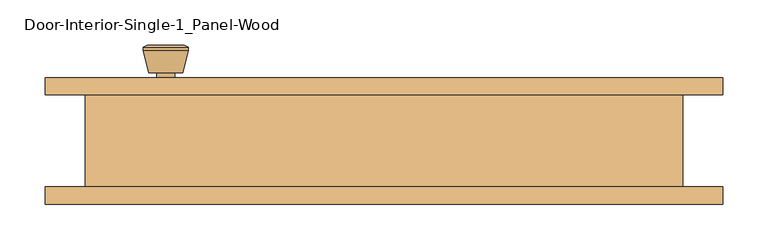
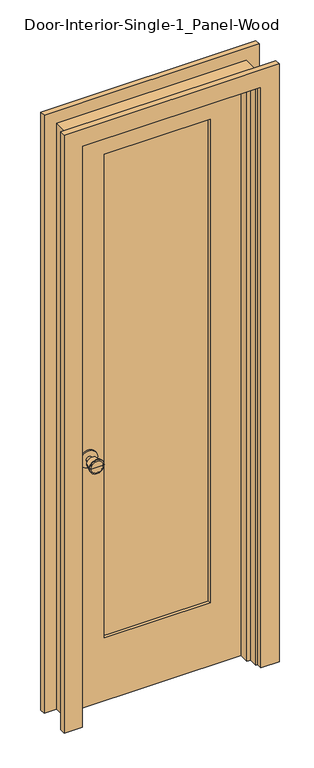
"""IFC4 building model written with IfcOpenShell, lengths in millimetres: door geometry, Door-Interior-Single-1_Panel-Wood."""

from ifc_helpers import new_model, si_unit, point, frame, frame_2d, origin, place, context, project, spatial, polyline, circle_curve, trimmed, segment, composite_curve, outline, extrude, faceted_brep, source, transform, mapped, element, save
from ifc_brep_helpers import plane_surface, cylinder_surface, revolved_surface, advanced_brep


def door_interior_single_1_panel_wood_33af59b7(model_context):
    return source(origin(), model_context, "Body", "SolidModel", [
        advanced_brep(
        [(-241.3, 6.7, 914.4), (-231.3, 6.7, 914.4), (-251.3, 6.7, 914.4), (-220.8241324, -42.3, 914.4), (-241.3, -42.3, 914.4), (-261.7758676, -42.3, 914.4), (-216.3, -40.4721319, 914.4), (-266.3, -40.4721319, 914.4), (-216.3, -37.0084537, 914.4), (-266.3, -37.0084537, 914.4), (-222.663764, -12.3, 914.4), (-259.936236, -12.3, 914.4), (-231.3, -12.3, 914.4), (-251.3, -12.3, 914.4)],
        [
            (0, 1),
            (1, 2, circle_curve(frame((-241.3, 6.7, 914.4), z_axis=(0.0, 1.0, 0.0), x_axis=(-1.0, 0.0, 0.0)), 10.0)),
            (2, 0),
            (2, 1, circle_curve(frame((-241.3, 6.7, 914.4), z_axis=(0.0, 1.0, 0.0), x_axis=(-1.0, 0.0, 0.0)), 10.0)),
            (3, 4),
            (4, 5),
            (5, 3, circle_curve(frame((-241.3, -42.3, 914.4), z_axis=(0.0, -1.0, 0.0), x_axis=(-1.0, 0.0, 0.0)), 20.4758676)),
            (3, 5, circle_curve(frame((-241.3, -42.3, 914.4), z_axis=(0.0, -1.0, 0.0), x_axis=(-1.0, 0.0, 0.0)), 20.4758676)),
            (6, 3),
            (5, 7),
            (7, 6, circle_curve(frame((-241.3, -40.4721319, 914.4), z_axis=(0.0, -1.0, 0.0), x_axis=(-1.0, 0.0, 0.0)), 25.0)),
            (6, 7, circle_curve(frame((-241.3, -40.4721319, 914.4), z_axis=(0.0, -1.0, 0.0), x_axis=(-1.0, 0.0, 0.0)), 25.0)),
            (8, 6),
            (7, 9),
            (9, 8, circle_curve(frame((-241.3, -37.0084537, 914.4), z_axis=(0.0, -1.0, 0.0), x_axis=(-1.0, 0.0, 0.0)), 25.0)),
            (8, 9, circle_curve(frame((-241.3, -37.0084537, 914.4), z_axis=(0.0, -1.0, 0.0), x_axis=(-1.0, 0.0, 0.0)), 25.0)),
            (10, 8),
            (9, 11),
            (11, 10, circle_curve(frame((-241.3, -12.3, 914.4), z_axis=(0.0, -1.0, 0.0), x_axis=(-1.0, 0.0, 0.0)), 18.636236)),
            (10, 11, circle_curve(frame((-241.3, -12.3, 914.4), z_axis=(0.0, -1.0, 0.0), x_axis=(-1.0, 0.0, 0.0)), 18.636236)),
            (12, 10),
            (11, 13),
            (13, 12, circle_curve(frame((-241.3, -12.3, 914.4), z_axis=(0.0, -1.0, 0.0), x_axis=(-1.0, 0.0, 0.0)), 10.0)),
            (12, 13, circle_curve(frame((-241.3, -12.3, 914.4), z_axis=(0.0, -1.0, 0.0), x_axis=(-1.0, 0.0, 0.0)), 10.0)),
            (1, 12),
            (13, 2),
        ],
        [
            plane_surface(frame((-241.3, 6.7, 914.4), z_axis=(0.0, 1.0, 0.0), x_axis=(-1.0, 0.0, 0.0))),
            plane_surface(frame((-241.3, -42.3, 914.4), z_axis=(0.0, -1.0, 0.0), x_axis=(-1.0, 0.0, 0.0))),
            revolved_surface(polyline([(-261.7758676, -42.3, 914.4), (-266.3, -40.4721319, 914.4)]), (-241.3, 6.7, 914.4), (0.0, 1.0, 0.0)),
            cylinder_surface(frame((-241.3, 6.7, 914.4), z_axis=(0.0, 1.0, 0.0), x_axis=(-1.0, 0.0, 0.0)), 25.0),
            revolved_surface(polyline([(-266.3, -37.0084537, 914.4), (-259.936236, -12.3, 914.4)]), (-241.3, 6.7, 914.4), (0.0, 1.0, 0.0)),
            plane_surface(frame((-241.3, -12.3, 914.4), z_axis=(0.0, 1.0, 0.0), x_axis=(-1.0, 0.0, 0.0))),
            cylinder_surface(frame((-241.3, 6.7, 914.4), z_axis=(0.0, 1.0, 0.0), x_axis=(-1.0, 0.0, 0.0)), 10.0),
        ],
        [
            (0, [[1, 2, 3]]),
            (0, [[-3, 4, -1]]),
            (1, [[5, 6, 7]]),
            (1, [[-6, -5, 8]]),
            (2, [[9, -7, 10, 11]]),
            (2, [[-10, -8, -9, 12]]),
            (3, [[13, -11, 14, 15]]),
            (3, [[-14, -12, -13, 16]]),
            (4, [[17, -15, 18, 19]]),
            (4, [[-18, -16, -17, 20]]),
            (5, [[21, -19, 22, 23]]),
            (5, [[-22, -20, -21, 24]]),
            (6, [[25, -23, 26, -2]]),
            (6, [[-26, -24, -25, -4]]),
        ],
    ),
        extrude(outline(composite_curve([segment(trimmed(circle_curve(frame_2d((914.4, -241.3)), 30.0), [point((914.4, -271.3))], [point((914.4, -211.3))], False, "CARTESIAN"), True, "CONTINUOUS"), segment(trimmed(circle_curve(frame_2d((914.4, -241.3)), 30.0), [point((914.4, -211.3))], [point((914.4, -271.3))], False, "CARTESIAN"), True, "CONTINUOUS")], self_intersect=False)), frame((0.0, 6.7, 0.0), z_axis=(0.0, 1.0, 0.0), x_axis=(0.0, 0.0, 1.0)), (0.0, 0.0, 1.0), 6.0),
        advanced_brep(
        [(-241.3, 53.625, 914.4), (-251.3, 53.625, 914.4), (-231.3, 53.625, 914.4), (-220.8241324, 102.625, 914.4), (-261.7758676, 102.625, 914.4), (-241.3, 102.625, 914.4), (-216.3, 100.7971319, 914.4), (-266.3, 100.7971319, 914.4), (-216.3, 97.3334537, 914.4), (-266.3, 97.3334537, 914.4), (-222.663764, 72.625, 914.4), (-259.936236, 72.625, 914.4), (-231.3, 72.625, 914.4), (-251.3, 72.625, 914.4)],
        [
            (0, 1),
            (1, 2, circle_curve(frame((-241.3, 53.625, 914.4), z_axis=(0.0, -1.0, 0.0), x_axis=(-1.0, 0.0, 0.0)), 10.0)),
            (2, 0),
            (2, 1, circle_curve(frame((-241.3, 53.625, 914.4), z_axis=(0.0, -1.0, 0.0), x_axis=(-1.0, 0.0, 0.0)), 10.0)),
            (3, 4, circle_curve(frame((-241.3, 102.625, 914.4), z_axis=(0.0, 1.0, 0.0), x_axis=(-1.0, 0.0, 0.0)), 20.4758676)),
            (4, 5),
            (5, 3),
            (4, 3, circle_curve(frame((-241.3, 102.625, 914.4), z_axis=(0.0, 1.0, 0.0), x_axis=(-1.0, 0.0, 0.0)), 20.4758676)),
            (6, 7, circle_curve(frame((-241.3, 100.7971319, 914.4), z_axis=(0.0, 1.0, 0.0), x_axis=(-1.0, 0.0, 0.0)), 25.0)),
            (7, 4),
            (3, 6),
            (7, 6, circle_curve(frame((-241.3, 100.7971319, 914.4), z_axis=(0.0, 1.0, 0.0), x_axis=(-1.0, 0.0, 0.0)), 25.0)),
            (8, 9, circle_curve(frame((-241.3, 97.3334537, 914.4), z_axis=(0.0, 1.0, 0.0), x_axis=(-1.0, 0.0, 0.0)), 25.0)),
            (9, 7),
            (6, 8),
            (9, 8, circle_curve(frame((-241.3, 97.3334537, 914.4), z_axis=(0.0, 1.0, 0.0), x_axis=(-1.0, 0.0, 0.0)), 25.0)),
            (10, 11, circle_curve(frame((-241.3, 72.625, 914.4), z_axis=(0.0, 1.0, 0.0), x_axis=(-1.0, 0.0, 0.0)), 18.636236)),
            (11, 9),
            (8, 10),
            (11, 10, circle_curve(frame((-241.3, 72.625, 914.4), z_axis=(0.0, 1.0, 0.0), x_axis=(-1.0, 0.0, 0.0)), 18.636236)),
            (12, 13, circle_curve(frame((-241.3, 72.625, 914.4), z_axis=(0.0, 1.0, 0.0), x_axis=(-1.0, 0.0, 0.0)), 10.0)),
            (13, 11),
            (10, 12),
            (13, 12, circle_curve(frame((-241.3, 72.625, 914.4), z_axis=(0.0, 1.0, 0.0), x_axis=(-1.0, 0.0, 0.0)), 10.0)),
            (1, 13),
            (12, 2),
        ],
        [
            plane_surface(frame((-241.3, 53.625, 914.4), z_axis=(0.0, -1.0, 0.0), x_axis=(-1.0, 0.0, 0.0))),
            plane_surface(frame((-241.3, 102.625, 914.4), z_axis=(0.0, 1.0, 0.0), x_axis=(-1.0, 0.0, 0.0))),
            revolved_surface(polyline([(-261.7758676, 102.625, 914.4), (-266.3, 100.7971319, 914.4)]), (-241.3, 53.625, 914.4), (0.0, -1.0, 0.0)),
            cylinder_surface(frame((-241.3, 53.625, 914.4), z_axis=(0.0, -1.0, 0.0), x_axis=(-1.0, 0.0, 0.0)), 25.0),
            revolved_surface(polyline([(-266.3, 97.3334537, 914.4), (-259.936236, 72.625, 914.4)]), (-241.3, 53.625, 914.4), (0.0, -1.0, 0.0)),
            plane_surface(frame((-241.3, 72.625, 914.4), z_axis=(0.0, -1.0, 0.0), x_axis=(-1.0, 0.0, 0.0))),
            cylinder_surface(frame((-241.3, 53.625, 914.4), z_axis=(0.0, -1.0, 0.0), x_axis=(-1.0, 0.0, 0.0)), 10.0),
        ],
        [
            (0, [[1, 2, 3]]),
            (0, [[-3, 4, -1]]),
            (1, [[5, 6, 7]]),
            (1, [[8, -7, -6]]),
            (2, [[9, 10, -5, 11]]),
            (2, [[12, -11, -8, -10]]),
            (3, [[13, 14, -9, 15]]),
            (3, [[16, -15, -12, -14]]),
            (4, [[17, 18, -13, 19]]),
            (4, [[20, -19, -16, -18]]),
            (5, [[21, 22, -17, 23]]),
            (5, [[24, -23, -20, -22]]),
            (6, [[-2, 25, -21, 26]]),
            (6, [[-4, -26, -24, -25]]),
        ],
    ),
        extrude(outline(composite_curve([segment(trimmed(circle_curve(frame_2d((914.4, -241.3)), 30.0), [point((914.4, -271.3))], [point((914.4, -211.3))], False, "CARTESIAN"), True, "CONTINUOUS"), segment(trimmed(circle_curve(frame_2d((914.4, -241.3)), 30.0), [point((914.4, -211.3))], [point((914.4, -271.3))], False, "CARTESIAN"), True, "CONTINUOUS")], self_intersect=False)), frame((0.0, 47.625, 0.0), z_axis=(0.0, 1.0, 0.0), x_axis=(0.0, 0.0, 1.0)), (0.0, 0.0, 1.0), 6.0),
        faceted_brep([(330.2, 47.625, 0.0), (330.2, -53.975, 0.0), (304.8, -53.975, 0.0), (304.8, -22.225, 0.0), (292.1, -22.225, 0.0), (292.1, 12.7, 0.0), (304.8, 12.7, 0.0), (304.8, 47.625, 0.0), (330.2, 47.625, 2159.0), (330.2, -53.975, 2159.0), (-330.2, -53.975, 2159.0), (-330.2, -53.975, 0.0), (-304.8, -53.975, 0.0), (-304.8, -53.975, 2133.6), (304.8, -53.975, 2133.6), (304.8, -22.225, 2133.6), (-304.8, -22.225, 2133.6), (-304.8, -22.225, 0.0), (-292.1, -22.225, 0.0), (-292.1, -22.225, 2120.9), (292.1, -22.225, 2120.9), (292.1, 12.7, 2120.9), (-292.1, 12.7, 2120.9), (-292.1, 12.7, 0.0), (-304.8, 12.7, 0.0), (-304.8, 12.7, 2133.6), (304.8, 12.7, 2133.6), (304.8, 47.625, 2133.6), (-304.8, 47.625, 2133.6), (-304.8, 47.625, 0.0), (-330.2, 47.625, 0.0), (-330.2, 47.625, 2159.0)], [[[0, 1, 2, 3, 4, 5, 6, 7]], [[1, 0, 8, 9]], [[2, 1, 9, 10, 11, 12, 13, 14]], [[3, 2, 14, 15]], [[4, 3, 15, 16, 17, 18, 19, 20]], [[5, 4, 20, 21]], [[6, 5, 21, 22, 23, 24, 25, 26]], [[7, 6, 26, 27]], [[0, 7, 27, 28, 29, 30, 31, 8]], [[9, 8, 31, 10]], [[15, 14, 13, 16]], [[21, 20, 19, 22]], [[27, 26, 25, 28]], [[30, 29, 24, 23, 18, 17, 12, 11]], [[10, 31, 30, 11]], [[16, 13, 12, 17]], [[22, 19, 18, 23]], [[28, 25, 24, 29]]]),
        extrude(outline(polyline([(2133.6, -304.8), (0.0, -304.8), (0.0, 304.8), (2133.6, 304.8), (2133.6, -304.8)]), holes=[polyline([(2014.5375, -184.15), (2014.5375, 184.15), (231.775, 184.15), (231.775, -184.15), (2014.5375, -184.15)])]), frame((0.0, 12.7, 0.0), z_axis=(0.0, 1.0, 0.0), x_axis=(0.0, 0.0, 1.0)), (0.0, 0.0, 1.0), 34.925),
        extrude(outline(polyline([(184.15, 24.3416667), (-184.15, 24.3416667), (-184.15, 35.9833333), (184.15, 35.9833333), (184.15, 24.3416667)])), frame((0.0, 0.0, 231.775), z_axis=(0.0, 0.0, 1.0), x_axis=(1.0, 0.0, 0.0)), (0.0, 0.0, 1.0), 1782.7625),
        extrude(outline(polyline([(0.0, 311.15), (0.0, 374.65), (2203.45, 374.65), (2203.45, -374.65), (0.0, -374.65), (0.0, -311.15), (2139.95, -311.15), (2139.95, 311.15), (0.0, 311.15)])), frame((0.0, 47.625, 0.0), z_axis=(0.0, 1.0, 0.0), x_axis=(0.0, 0.0, 1.0)), (0.0, 0.0, 1.0), 19.05),
        extrude(outline(polyline([(0.0, 311.15), (0.0, 374.65), (2203.45, 374.65), (2203.45, -374.65), (0.0, -374.65), (0.0, -311.15), (2139.95, -311.15), (2139.95, 311.15), (0.0, 311.15)])), frame((0.0, -73.025, 0.0), z_axis=(0.0, 1.0, 0.0), x_axis=(0.0, 0.0, 1.0)), (0.0, 0.0, 1.0), 19.05),
    ])


if __name__ == "__main__":
    model = new_model("IFC4")
    model_context = context("Model", 3, world=origin())
    ifc_project = project(units=[si_unit("LENGTHUNIT", "METRE", prefix="MILLI")], contexts=[model_context])
    site = spatial("IfcSite", under=ifc_project)
    building = spatial("IfcBuilding", under=site)
    placement = place(None, origin())
    door_interior_single_1_panel_wood_shape = door_interior_single_1_panel_wood_33af59b7(model_context)
    element("IfcDoor", 1, ObjectType="Door-Interior-Single-1_Panel-Wood", at=placement, inside=building, context=model_context, shape_type="MappedRepresentation", body=[
        mapped(door_interior_single_1_panel_wood_shape, transform((0.0, 0.0, 0.0), x_axis=(1.0, 0.0, 0.0), y_axis=(0.0, 1.0, 0.0), z_axis=(0.0, 0.0, 1.0))),
    ])
    save(model, "model.ifc")

# Revit data of these elements
# Type "Door-Interior-Single-1_Panel-Wood"
#   Type Mark = "12"
#   Assembly Code = "C1020300"
#   Analytic Construction = "Wooden"
#   Top Rail = 0' - 4 11/16"
#   Thickness = 0' - 1 3/8"
#   Thermal Resistance (R) = 2.5876 (h·ft²·°F)/BTU
#   Swing Angle [instance default] = 90.00°
#   Stiles = 0' - 4 3/4"
#   Rough Width = 2' - 2"
#   Rough Height = 7' - 1"
#   Height = 7' - 0"
#   Width = 2' - 0"
#   Heat Transfer Coefficient (U) = 0.3865 BTU/(h·ft²·°F)
#   Bottom Rail = 0' - 9 1/8"
#   Trim Material = Cherry
#   Panel Material = Cherry
#   Frame Material = Cherry
#   Door Handle Material = Aluminum
#   Visual Light Transmittance = 0
#   Solar Heat Gain Coefficient = 0
#   Wall Closure = (empty or 0)
#   Function = (empty or 0)
# Element 1 (IfcDoor, "Door-Interior-Single-1_Panel-Wood")
#   Materials on its faces: "Cherry", "Aluminum"
# Materials
#   "Cherry": class "Wood", colour RGB 226 177 128, transparency 0, Description = "Prunus Serotina", Cost = 0
#   "Aluminum": class "Metal", colour RGB 247 247 247, transparency 0, Description = "Aluminum 6061", Cost = 0
